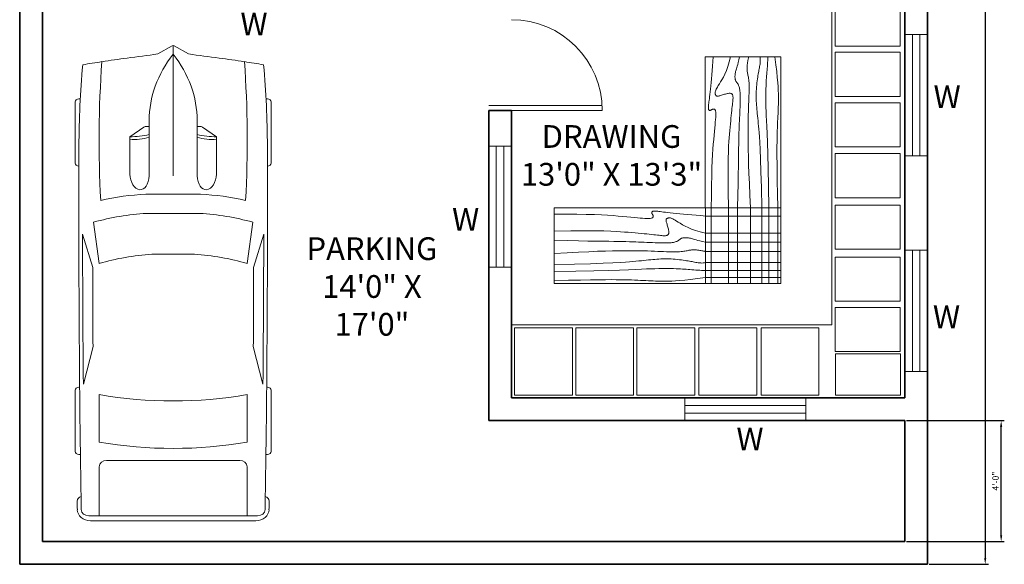
# Model space of a CAD drawing. Units: inches. Extents: x 1642 to 5612, y 1595 to 4064.
# Tile 1 of 6: x 1675 to 2066, y 1595 to 1811. Entities that reach past the tile are written whole.
import ezdxf

# ---------------------------------------------------------------- set-up
doc = ezdxf.new("R2010")
doc.units = ezdxf.units.IN
for name, color, linetype, lineweight in [('A-ANNO-DIMS', 2, 'Continuous', 18), ('A-ANNO-TEXT', 7, 'Continuous', 18), ('A-AREA-IDEN', 7, 'Continuous', 25), ('A-DOOR', 3, 'Continuous', 18), ('A-EQPM', 8, 'Continuous', 13), ('A-FURN', 8, 'Continuous', 13), ('A-GLAZ', 4, 'Continuous', 18), ('A-WALL', 7, 'Continuous', 35)]:
    doc.layers.add(name, color=color, linetype=linetype, lineweight=lineweight)
doc.styles.get("Standard").update_dxf_attribs({"font": 'arial.ttf'})
doc.dimstyles.new('ISO-25', dxfattribs={"dimtxt": 2.5, "dimasz": 2.5, "dimexe": 1.25, "dimexo": 0.625, "dimtad": 1, "dimdec": 0, "dimlunit": 3, "dimtxsty": 'Standard', "dimcen": 2.5, "dimadec": 0, "dimazin": 0, "dimtfac": 1, "dimtdec": 0, "dimtmove": 0, "dimatfit": 3, "dimfxl": 1, "dimarcsym": 0})

# ---------------------------------------------------------------- blocks, each defined once
blk = doc.blocks.new('Table - Rectangular Woodgrain 60 x 30 in.')
for p, q in [((0, 0), (0, -30)), ((60, 0), (0, 0)), ((60, -30), (60, 0)), ((0, -30), (60, -30))]:
    blk.add_line(p, q)
for points in [[(0, -2.4), (4.8155, -2.418), (9.0302, -2.4688), (12.709, -2.5477), (15.9167, -2.65), (18.7181, -2.7711), (21.1781, -2.9063), (23.3616, -3.0508), (25.3333, -3.2), (27.1477, -3.3495), (28.8172, -3.4958), (30.3437, -3.636), (31.7291, -3.7667), (32.9756, -3.8849), (34.0849, -3.9875), (35.059, -4.0714), (35.9, -4.1334), (36.6114, -4.1711), (37.2041, -4.1854), (37.6906, -4.1779), (38.0833, -4.15), (38.3948, -4.1034), (38.6375, -4.0396), (38.8239, -3.9602), (38.9666, -3.8667), (39.0764, -3.7608), (39.1573, -3.6448), (39.2116, -3.521), (39.2416, -3.3917), (39.2498, -3.2593), (39.2385, -3.1261), (39.21, -2.9944), (39.1666, -2.8667), (39.111, -2.7447), (39.0468, -2.6281), (38.978, -2.5163), (38.9083, -2.4083), (38.8418, -2.3035), (38.7823, -2.201), (38.7337, -2.1001), (38.7, -2), (38.6844, -1.9003), (38.6875, -1.8021), (38.7094, -1.707), (38.75, -1.6167), (38.8094, -1.5326), (38.8875, -1.4563), (38.9844, -1.3893), (39.1, -1.3333), (39.2351, -1.2896), (39.3937, -1.2583), (39.5804, -1.2396), (39.8, -1.2333), (40.057, -1.2396), (40.3562, -1.2583), (40.7023, -1.2896), (41.1, -1.3333), (41.5547, -1.3895), (42.0755, -1.4573), (42.6721, -1.5361), (43.3542, -1.625), (44.1316, -1.7233), (45.014, -1.8302), (46.0114, -1.9449), (47.1333, -2.0667), (48.3862, -2.1947), (49.7625, -2.3281), (51.2513, -2.4663), (52.8416, -2.6083), (54.5226, -2.7535), (56.2833, -2.9011), (58.1127, -3.0501), (60, -3.2)], [(0, -9.2), (6.5759, -9.0858), (11.9385, -9.0365), (16.2527, -9.0418), (19.6833, -9.0917), (22.3952, -9.1759), (24.5531, -9.2844), (26.322, -9.4069), (27.8666, -9.5333), (29.3241, -9.6553), (30.7203, -9.7719), (32.0532, -9.8837), (33.3208, -9.9917), (34.5213, -10.0965), (35.6526, -10.199), (36.7128, -10.2999), (37.7, -10.4), (38.6129, -10.4996), (39.4531, -10.5969), (40.223, -10.6895), (40.925, -10.775), (41.5613, -10.8512), (42.1344, -10.9156), (42.6465, -10.966), (43.1, -11), (43.4976, -11.0158), (43.8437, -11.0136), (44.143, -10.9942), (44.4, -10.9583), (44.6195, -10.9069), (44.8062, -10.8406), (44.9648, -10.7603), (45.1, -10.6667), (45.2155, -10.5598), (45.3114, -10.4365), (45.3871, -10.2929), (45.4416, -10.125), (45.4743, -9.929), (45.4844, -9.7011), (45.4709, -9.4371), (45.4333, -9.1333), (45.3716, -8.7883), (45.2896, -8.4104), (45.1919, -8.0107), (45.0833, -7.6), (44.9685, -7.1893), (44.8521, -6.7896), (44.7388, -6.4117), (44.6333, -6.0667), (44.54, -5.7628), (44.4614, -5.4979), (44.4001, -5.2675), (44.3583, -5.0667), (44.3384, -4.8909), (44.3427, -4.7354), (44.3736, -4.5956), (44.4333, -4.4667), (44.5236, -4.3453), (44.6427, -4.2333), (44.7884, -4.1339), (44.9583, -4.05), (45.1501, -3.9849), (45.3614, -3.9417), (45.59, -3.9234), (45.8333, -3.9333), (46.0915, -3.9749), (46.3734, -4.0531), (46.6906, -4.1736), (47.0542, -4.3417), (47.4756, -4.5629), (47.9661, -4.8427), (48.5372, -5.1866), (49.2, -5.6), (49.9676, -6.0844), (50.8594, -6.625), (51.8965, -7.2031), (53.1, -7.8), (54.491, -8.3969), (56.0906, -8.975), (57.9199, -9.5156), (60, -10)], [(0, -12.8), (5.1847, -12.9322), (9.6213, -13.0323), (13.3963, -13.1059), (16.5958, -13.1583), (19.3063, -13.1952), (21.614, -13.2219), (23.6054, -13.2439), (25.3666, -13.2667), (26.9728, -13.2947), (28.4531, -13.3281), (29.8256, -13.3663), (31.1083, -13.4083), (32.3191, -13.4535), (33.476, -13.501), (34.597, -13.5501), (35.7, -13.6), (36.7984, -13.6497), (37.8875, -13.6979), (38.9578, -13.743), (40, -13.7833), (41.0047, -13.8174), (41.9625, -13.8438), (42.864, -13.8607), (43.7, -13.8667), (44.4631, -13.8604), (45.1552, -13.8417), (45.7801, -13.8104), (46.3416, -13.7667), (46.8439, -13.7104), (47.2906, -13.6417), (47.6858, -13.5604), (48.0333, -13.4667), (48.3375, -13.3608), (48.6042, -13.2448), (48.8396, -13.121), (49.05, -12.9917), (49.2417, -12.8593), (49.4208, -12.7261), (49.5937, -12.5944), (49.7667, -12.4667), (49.9452, -12.3451), (50.1323, -12.2313), (50.3303, -12.1268), (50.5416, -12.0333), (50.7686, -11.9524), (51.0135, -11.8854), (51.2788, -11.8341), (51.5666, -11.8), (51.8785, -11.7843), (52.2116, -11.7865), (52.562, -11.8059), (52.926, -11.8417), (53.2998, -11.8931), (53.6795, -11.9594), (54.0614, -12.0397), (54.4416, -12.1333), (54.8223, -12.2401), (55.2293, -12.3625), (55.6942, -12.5037), (56.2489, -12.6667), (56.9251, -12.8547), (57.7545, -13.0708), (58.7689, -13.3182), (60, -13.6)], [(0, -18), (5.124, -17.7273), (9.6609, -17.5057), (13.6705, -17.3303), (17.2125, -17.1958), (20.3467, -17.0973), (23.1328, -17.0297), (25.6307, -16.9878), (27.9, -16.9667), (29.9928, -16.9617), (31.9302, -16.9703), (33.7254, -16.9907), (35.3917, -17.0208), (36.9423, -17.0588), (38.3906, -17.1026), (39.7499, -17.1503), (41.0333, -17.2), (42.2519, -17.2496), (43.4073, -17.2969), (44.4986, -17.3395), (45.525, -17.375), (46.4858, -17.4012), (47.3802, -17.4156), (48.2074, -17.416), (48.9667, -17.4), (49.6583, -17.3662), (50.2872, -17.3167), (50.8595, -17.2547), (51.3812, -17.1833), (51.8584, -17.1057), (52.2971, -17.025), (52.7034, -16.9443), (53.0833, -16.8667), (53.443, -16.7951), (53.789, -16.7313), (54.128, -16.6768), (54.4666, -16.6334), (54.8115, -16.6024), (55.1693, -16.5854), (55.5465, -16.5841), (55.95, -16.6), (56.3828, -16.6337), (56.8346, -16.6823), (57.2915, -16.7418), (57.7396, -16.8084), (58.165, -16.878), (58.5539, -16.9469), (58.8924, -17.0111), (59.1666, -17.0667), (59.3679, -17.1107), (59.5078, -17.1438), (59.6032, -17.1675), (59.6708, -17.1833), (59.7275, -17.193), (59.7901, -17.1979), (59.8753, -17.1998), (60, -17.2)], [(0, -22.4), (8.0098, -22.2501), (14.4094, -22.1011), (19.4168, -21.9535), (23.25, -21.8083), (26.1269, -21.6663), (28.2656, -21.5281), (29.884, -21.3947), (31.2, -21.2667), (32.3967, -21.1448), (33.5172, -21.0292), (34.5697, -20.9198), (35.5625, -20.8167), (36.5037, -20.7198), (37.4015, -20.6292), (38.2642, -20.5448), (39.1, -20.4667), (39.9164, -20.3951), (40.7187, -20.3313), (41.5117, -20.2768), (42.3, -20.2333), (43.0883, -20.2024), (43.8812, -20.1854), (44.6836, -20.1841), (45.5, -20.2), (46.3328, -20.234), (47.1747, -20.2844), (48.0163, -20.3488), (48.8479, -20.425), (49.66, -20.5106), (50.4429, -20.6031), (51.1872, -20.7004), (51.8833, -20.8), (52.5246, -20.8999), (53.1166, -20.9995), (53.6681, -21.0983), (54.1875, -21.1958), (54.6834, -21.2919), (55.1646, -21.3859), (55.6394, -21.4777), (56.1167, -21.5667), (56.6028, -21.6515), (57.0961, -21.7266), (57.5929, -21.7852), (58.0896, -21.8208), (58.5823, -21.8268), (59.0674, -21.7964), (59.5412, -21.723), (60, -21.6)], [(0, -25.2), (8.6355, -25.0504), (15.7026, -24.9031), (21.4049, -24.7606), (25.9458, -24.625), (29.529, -24.4988), (32.3578, -24.3844), (34.6359, -24.284), (36.5667, -24.2), (38.3213, -24.1341), (39.9417, -24.0854), (41.437, -24.0523), (42.8167, -24.0333), (44.0901, -24.0268), (45.2667, -24.0313), (46.3557, -24.0451), (47.3667, -24.0667), (48.309, -24.0947), (49.1928, -24.1287), (50.0284, -24.168), (50.826, -24.2125), (51.5959, -24.2617), (52.3483, -24.3151), (53.0935, -24.3725), (53.8417, -24.4334), (54.6009, -24.497), (55.3699, -24.561), (56.1454, -24.6226), (56.9239, -24.6792), (57.7021, -24.7279), (58.4764, -24.7662), (59.2435, -24.7911), (60, -24.8)], [(0, -28.8), (5.6867, -28.6681), (10.45, -28.5698), (14.407, -28.5012), (17.675, -28.4584), (20.3711, -28.4374), (22.6125, -28.4344), (24.5164, -28.4455), (26.2, -28.4667), (27.762, -28.4947), (29.2276, -28.5281), (30.6033, -28.5663), (31.8958, -28.6084), (33.1118, -28.6535), (34.2578, -28.7011), (35.3405, -28.7501), (36.3666, -28.8), (37.3443, -28.8497), (38.288, -28.8974), (39.2137, -28.9412), (40.1375, -28.9792), (41.0753, -29.0093), (42.0432, -29.0297), (43.0572, -29.0384), (44.1333, -29.0333), (45.2936, -29.0114), (46.5843, -28.9641), (48.0579, -28.8816), (49.7666, -28.7542), (51.7629, -28.5721), (54.0989, -28.3255), (56.8272, -28.0048), (60, -27.6)]]:
    blk.add_lwpolyline(points)
blk = doc.blocks.new('*D11')
at = {"layer": 'A-ANNO-DIMS', "color": 0, "lineweight": -2, "transparency": 16777216}
for p, q in [((2035.91, 2134.99), (2059.41, 2134.99)), ((2058.16, 2132.49), (2058.16, 1597.49)), ((2035.91, 1594.99), (2059.41, 1594.99))]:
    blk.add_line(p, q, dxfattribs=at)
at = {"layer": 'A-ANNO-DIMS', "color": 0, "transparency": 16777216}
for points in [[(2057.74, 2132.49), (2058.57, 2132.49), (2058.16, 2134.99)], [(2057.74, 1597.49), (2058.57, 1597.49), (2058.16, 1594.99)]]:
    blk.add_solid(points, dxfattribs=at)
at = {"layer": 'Defpoints', "color": 0, "transparency": 16777216}
for p in [(2035.28, 2134.99), (2035.28, 1594.99), (2058.16, 1594.99)]:
    blk.add_point(p, dxfattribs=at)
at = {"layer": 'A-ANNO-DIMS', "color": 0, "transparency": 16777216, "insert": (2056.26, 1864.99), "char_height": 2.5, "width": 4.3062, "attachment_point": 5, "rotation": 90}
blk.add_mtext("45'", dxfattribs=at)
blk = doc.blocks.new('*U13')
for p, q in [((21.1, 37.41), (21.1, 36.83)), ((46.55, 38.89), (22.35, 38.89)), ((47.8, 37.39), (47.8, 37.41)), ((87.99, 31.87), (74.76, 35.92)), ((134.31, 35.6), (119.29, 31.78)), ((135.45, 37.07), (135.45, 37.41)), ((136.7, 38.89), (160.9, 38.89)), ((162.15, 37.41), (162.15, 36.77)), ((70.03, 31.54), (86.41, 29.35)), ((186.47, -33.5), (186.47, 33.5)), ((188.4, -32.76), (188.4, 32.76)), ((138.42, 29.35), (157.25, 29.35)), ((186.47, 29.35), (167.01, 29.35)), ((164.52, 26.39), (164.52, -26.39)), ((32.27, 11.63), (36.13, 17.17)), ((36.13, 17.17), (50.94, 17.17)), ((29.77, 9.51), (51.68, 9.51)), ((32.12, 9.51), (32.12, 11.15)), ((58.92, -10.77), (58.92, 10.77)), ((66.55, -10.53), (66.55, 10.53)), ((82.74, 8.5), (82.74, -8.5)), ((186.47, -10.53), (186.47, 10.53)), ((3.27, 6.13), (0.1, 0.41)), ((0, 0), (51.68, 0)), ((0.1, -0.41), (3.27, -6.13)), ((29.77, -9.51), (51.68, -9.51)), ((32.12, -9.51), (32.12, -11.15)), ((32.27, -11.63), (36.13, -17.17)), ((36.13, -17.17), (50.94, -17.17)), ((86.41, -29.35), (70.03, -31.54)), ((157.25, -29.35), (138.42, -29.35)), ((167.01, -29.35), (186.47, -29.35)), ((87.99, -31.87), (74.76, -35.92)), ((134.31, -35.6), (119.29, -31.78)), ((21.1, -37.41), (21.1, -36.83)), ((46.55, -38.89), (22.35, -38.89)), ((47.8, -37.39), (47.8, -37.41)), ((135.45, -37.07), (135.45, -37.41)), ((136.7, -38.89), (160.9, -38.89)), ((162.15, -37.41), (162.15, -36.77))]:
    blk.add_line(p, q)
for centre, major_axis, ratio, start_param, end_param in [((266.03, -27.52), (0, 313.31), 0.842304, 1.367076, 1.39176), ((41.19, -490.86), (0, 528.23), 0.842304, 0.00281, 0.075598), ((22.35, 37.41), (0, -1.48), 0.842304, 3.141593, 4.712389), ((64.48, -10555.62), (0, 10593.03), 0.842304, -0.013397, 0.002797), ((46.55, 37.41), (0, 1.48), 0.842304, -1.570796, 0), ((64.48, -10555.62), (0, -10591.55), 0.842304, 3.133765, 3.140441), ((136.7, 37.41), (0, -1.48), 0.842304, 3.141593, 4.712389), ((160.9, 37.41), (0, 1.48), 0.842304, -1.570796, 0), ((180.63, 35.84), (0, 2.22), 0.842304, -0.013017, 1.249894), ((64.48, -10556.36), (0, 10595.31), 0.842304, -0.013397, -0.013017), ((183.98, 33.5), (0, -2.96), 0.842304, 1.570796, 3.128196), ((183.98, 32.76), (0, -5.25), 0.842304, 1.570796, 3.128196), ((135.29, 5.39), (0, 81.77), 0.842304, 1.245306, 1.50788), ((95.79, -3666.35), (0, -3698.24), 0.842304, 3.134049, 3.144098), ((259.18, -27.52), (0, -305.3), 0.842304, 4.528606, 4.561838), ((37.47, -593.96), (0, -623.33), 0.842304, 3.096046, 3.200911), ((134.4, 5.39), (0, -89.78), 0.842304, 4.449482, 4.652344), ((149.6, 2.8), (0, -79.58), 0.842304, 4.372215, 4.640744), ((17.08, 0), (0, 147.02), 0.842304, 4.511394, 4.913384), ((35.91, 0), (0, 147.02), 0.842304, 4.511394, 4.913384), ((167.01, 26.39), (0, 2.96), 0.842304, 0, 1.570796), ((-204.49, 52.4), (0, -250.96), 0.842304, 1.385369, 1.434372), ((13.04, 17.01), (0, 27.42), 0.842304, 4.435146, 4.718221), ((14.2, 17.01), (0, 27.42), 0.842304, 4.435146, 4.718221), ((50.79, 13.34), (6.34, -0.36), 0.603834, -1.395552, 1.581315), ((29.77, -46.66), (0, 56.17), 0.842304, 0, 0.590319), ((32.75, 11.15), (0, 0.74), 0.842304, 0.879714, 1.570796), ((0.62, 0), (0, -0.74), 0.842304, 4.131459, 5.293319), ((29.77, 46.66), (0, 56.17), 0.842304, 2.551274, 3.141593), ((-204.49, -52.4), (0, 250.96), 0.842304, -1.434372, -1.385369), ((32.75, -11.15), (0, -0.74), 0.842304, 4.712389, 5.403472), ((13.04, -17.01), (0, -27.42), 0.842304, 1.564964, 1.848039), ((14.2, -17.01), (0, -27.42), 0.842304, 1.564964, 1.848039), ((134.4, -5.39), (0, -89.78), 0.842304, -1.510751, -1.307889), ((135.29, -5.39), (0, -81.77), 0.842304, -1.50788, -1.245306), ((149.6, -2.8), (0, -79.58), 0.842304, -1.499151, -1.230623), ((259.18, 27.52), (0, 305.3), 0.842304, 1.721348, 1.754579), ((167.01, -26.39), (0, -2.96), 0.842304, 4.712389, 6.283185), ((266.03, 27.52), (0, 313.31), 0.842304, 1.749832, 1.774517), ((37.47, 593.96), (0, -623.33), 0.842304, -0.059319, 0.045547), ((95.79, 3666.35), (0, -3698.24), 0.842304, -0.002505, 0.007544), ((183.98, -33.5), (0, 2.96), 0.842304, 3.15499, 4.712389), ((183.98, -32.76), (0, -5.25), 0.842304, 0.013397, 1.570796), ((41.19, 490.86), (0, -528.23), 0.842304, -0.075598, -0.00281), ((22.35, -37.41), (0, 1.48), 0.842304, 1.570796, 3.141593), ((64.48, 10555.62), (0, 10593.03), 0.842304, 3.138796, 3.15499), ((46.55, -37.41), (0, -1.48), 0.842304, 0, 1.570796), ((64.48, 10555.62), (0, -10591.55), 0.842304, 0.001152, 0.007828), ((136.7, -37.41), (0, -1.48), 0.842304, -1.570796, 0), ((160.9, -37.41), (0, 1.48), 0.842304, 3.141593, 4.712389), ((180.63, -35.84), (0, -2.22), 0.842304, -1.249894, 0.013017), ((64.48, 10556.36), (0, 10595.31), 0.842304, 3.15461, 3.15499)]:
    blk.add_ellipse(centre, major_axis=major_axis, ratio=ratio, start_param=start_param, end_param=end_param)
at = {"extrusion": (0, 0, -1)}
blk.add_ellipse((50.79, -13.34), major_axis=(6.34, 0.36), ratio=0.603834, start_param=-1.395552, end_param=1.581315, dxfattribs=at)
blk = doc.blocks.new('WIN-48x9')
for p, q in [((0, 48), (0, 0)), ((9, 48), (0, 48)), ((3, 48), (3, 0)), ((6, 0), (6, 48)), ((9, 0), (9, 48)), ((0, 0), (9, 0))]:
    blk.add_line(p, q)
blk = doc.blocks.new('DOOR-SWING-36')
for p, q in [((36, 2), (0, 2)), ((36, 0), (0, 0))]:
    blk.add_line(p, q)
blk.add_arc((36, 0), 36, 90, 180)
blk = doc.blocks.new('SEATING-CUSHION-NARROW')
blk.add_lwpolyline([(0, 17.53), (25.79, 17.53), (25.79, 0), (0, 0)], close=True)
blk = doc.blocks.new('SEATING-CUSHION-WIDE')
blk.add_lwpolyline([(0, 26.61), (22.95, 26.61), (22.95, 0), (0, 0)], close=True)
blk = doc.blocks.new('SEATING-CUSHION-END')
blk.add_line((0, 0), (25.79, 0))
blk.add_lwpolyline([(0, 0), (0, 16.43), (25.79, 16.43), (25.79, 0)])
blk = doc.blocks.new('*D64')
at = {"layer": 'A-ANNO-DIMS', "color": 0, "lineweight": -2, "transparency": 16777216}
for p, q in [((2026.91, 1651.99), (2065.73, 1651.99)), ((2064.48, 1606.49), (2064.48, 1649.49)), ((2026.91, 1603.99), (2065.73, 1603.99))]:
    blk.add_line(p, q, dxfattribs=at)
at = {"layer": 'A-ANNO-DIMS', "color": 0, "transparency": 16777216}
for points in [[(2064.06, 1649.49), (2064.9, 1649.49), (2064.48, 1651.99)], [(2064.06, 1606.49), (2064.9, 1606.49), (2064.48, 1603.99)]]:
    blk.add_solid(points, dxfattribs=at)
at = {"layer": 'Defpoints', "color": 0, "transparency": 16777216}
for p in [(2026.28, 1651.99), (2064.48, 1651.99), (2026.28, 1603.99)]:
    blk.add_point(p, dxfattribs=at)
at = {"layer": 'A-ANNO-DIMS', "color": 0, "transparency": 16777216, "insert": (2062.58, 1627.99), "char_height": 2.5, "attachment_point": 5, "rotation": 90}
blk.add_mtext('4\'-0"', dxfattribs=at)

msp = doc.modelspace()

# ---------------------------------------------------------------- linework, layer by layer
at = {"layer": 'A-DOOR'}
msp.add_line((1861.28, 1776.99), (1870.28, 1776.99), dxfattribs=at)
at = {"layer": 'A-FURN'}
for p, q in [((1997.28, 1819.99), (1997.28, 1689.99)), ((1956.34, 1736.32), (1956.34, 1706.32)), ((1959.94, 1736.32), (1959.94, 1706.32)), ((1965.14, 1736.32), (1965.14, 1706.32)), ((1969.54, 1736.32), (1969.54, 1706.32)), ((1972.34, 1736.32), (1972.34, 1706.32)), ((1975.94, 1736.32), (1975.94, 1706.32)), ((1977.14, 1736.32), (1977.14, 1706.32)), ((1947.24, 1733.12), (1977.14, 1733.12)), ((1947.24, 1726.32), (1977.14, 1726.32)), ((1947.24, 1722.72), (1977.14, 1722.72)), ((1947.24, 1719.12), (1977.14, 1719.12)), ((1947.24, 1714.72), (1977.14, 1714.72)), ((1947.24, 1711.52), (1977.14, 1711.52)), ((1947.24, 1708.72), (1977.14, 1708.72)), ((1947.24, 1706.32), (1977.14, 1706.32)), ((1870.28, 1689.99), (1997.28, 1689.99))]:
    msp.add_line(p, q, dxfattribs=at)
for points in [[(1949.54, 1736.32), (1949.54, 1706.32)], [(2024.55, 1660.99), (1998.76, 1660.99)]]:
    msp.add_lwpolyline(points, dxfattribs=at)
at = {"layer": 'A-WALL'}
for p, q in [((1675.28, 1594.99), (1675.28, 2134.99)), ((2035.28, 2134.99), (2035.28, 1594.99)), ((2026.28, 1819.99), (2026.28, 1660.99)), ((1684.28, 1603.99), (1684.28, 1816.99)), ((1870.28, 1774.99), (1861.28, 1774.99)), ((1861.28, 1774.99), (1870.28, 1774.99)), ((1861.28, 1774.99), (1861.28, 1660.99)), ((1870.28, 1774.99), (1870.28, 1660.99)), ((1861.28, 1660.99), (1861.28, 1651.99)), ((1870.28, 1660.99), (2026.28, 1660.99)), ((1864.28, 1651.99), (1861.28, 1651.99)), ((1864.28, 1651.99), (2026.28, 1651.99)), ((2026.28, 1651.99), (2026.28, 1603.99)), ((2026.28, 1603.99), (1684.28, 1603.99)), ((2035.28, 1594.99), (1675.28, 1594.99))]:
    msp.add_line(p, q, dxfattribs=at)

# ---------------------------------------------------------------- block references
at = {"layer": 'A-DOOR', "extrusion": (0, 0, -1), "zscale": -1}
msp.add_blockref('DOOR-SWING-36', (-1906.28, 1774.99), dxfattribs=at)
at = {"layer": 'A-EQPM', "rotation": 270}
msp.add_blockref('*U13', (1736.14, 1800.7), dxfattribs=at)
at = {"layer": 'A-FURN'}
for name, p in [('SEATING-CUSHION-NARROW', (1998.68, 1800.43)), ('SEATING-CUSHION-NARROW', (1998.68, 1780.54)), ('SEATING-CUSHION-NARROW', (1998.68, 1760.52)), ('SEATING-CUSHION-NARROW', (1998.68, 1740.35)), ('Table - Rectangular Woodgrain 60 x 30 in.', (1887.24, 1736.32)), ('SEATING-CUSHION-NARROW', (1998.68, 1719.95)), ('SEATING-CUSHION-NARROW', (1998.68, 1699.32)), ('SEATING-CUSHION-NARROW', (1998.68, 1679.38)), ('SEATING-CUSHION-WIDE', (1871.55, 1662.14)), ('SEATING-CUSHION-WIDE', (1895.76, 1662.14)), ('SEATING-CUSHION-WIDE', (1920, 1662.14)), ('SEATING-CUSHION-WIDE', (1944.58, 1662.14)), ('SEATING-CUSHION-WIDE', (1969.29, 1662.14)), ('SEATING-CUSHION-END', (1998.76, 1662.09))]:
    msp.add_blockref(name, p, dxfattribs=at)
at = {"layer": 'A-FURN', "rotation": 90}
msp.add_blockref('Table - Rectangular Woodgrain 60 x 30 in.', (1947.14, 1736.32), dxfattribs=at)
at = {"layer": 'A-GLAZ'}
for p in [(2026.28, 1757.06), (1861.28, 1712.89), (2026.28, 1671.52)]:
    msp.add_blockref('WIN-48x9', p, dxfattribs=at)
at = {"layer": 'A-GLAZ', "rotation": 269.9999999999998}
msp.add_blockref('WIN-48x9', (1939.06, 1660.99), dxfattribs=at)

# ---------------------------------------------------------------- texts
at = {"layer": 'A-ANNO-TEXT', "char_height": 9, "attachment_point": 1}
for insert in [(1706.8, 1813.76), (1981.66, 1784.91), (1790.73, 1736.32), (1981.42, 1697.64), (1903.49, 1649.25)]:
    msp.add_mtext_dynamic_manual_height_columns('\\pxqc;W', width=122.7897, gutter_width=12.5, heights=[0], dxfattribs=dict(at, insert=insert))
at = {"layer": 'A-AREA-IDEN', "char_height": 9, "attachment_point": 1}
for s, width, insert in [('\\pxqc;DRAWING\\P13\'0" X 13\'3"', 74.6356, (1872.66, 1769.17)), ('\\pxqc;PARKING\\P14\'0" X 17\'0"', 69.783, (1780.07, 1724.68))]:
    msp.add_mtext_dynamic_manual_height_columns(s, width=width, gutter_width=12.5, heights=[0], dxfattribs=dict(at, insert=insert))

# ---------------------------------------------------------------- dimensions: what is measured, and where the dimension line sits
at = {"layer": 'A-ANNO-DIMS'}
for base, p1, p2, override, picture, middle in [((2058.16, 1594.99), (2035.28, 2134.99), (2035.28, 1594.99), {"dimclrd": 0, "dimclre": 0, "dimclrt": 0}, '*D11', (2056.26, 1864.99)), ((2064.48, 1651.99), (2026.28, 1603.99), (2026.28, 1651.99), {"dimdec": 1, "dimlfac": 1, "dimrnd": 0, "dimzin": 1, "dimdsep": 46, "dimlunit": 4, "dimfrac": 2}, '*D64', (2062.58, 1627.99))]:
    dim = msp.add_linear_dim(base=base, p1=p1, p2=p2, angle=90, dimstyle='ISO-25', override=override, dxfattribs=at)
    dim.commit()
    dim.dimension.update_dxf_attribs({"geometry": picture, "text_midpoint": middle})

doc.saveas('drawing.dxf')
